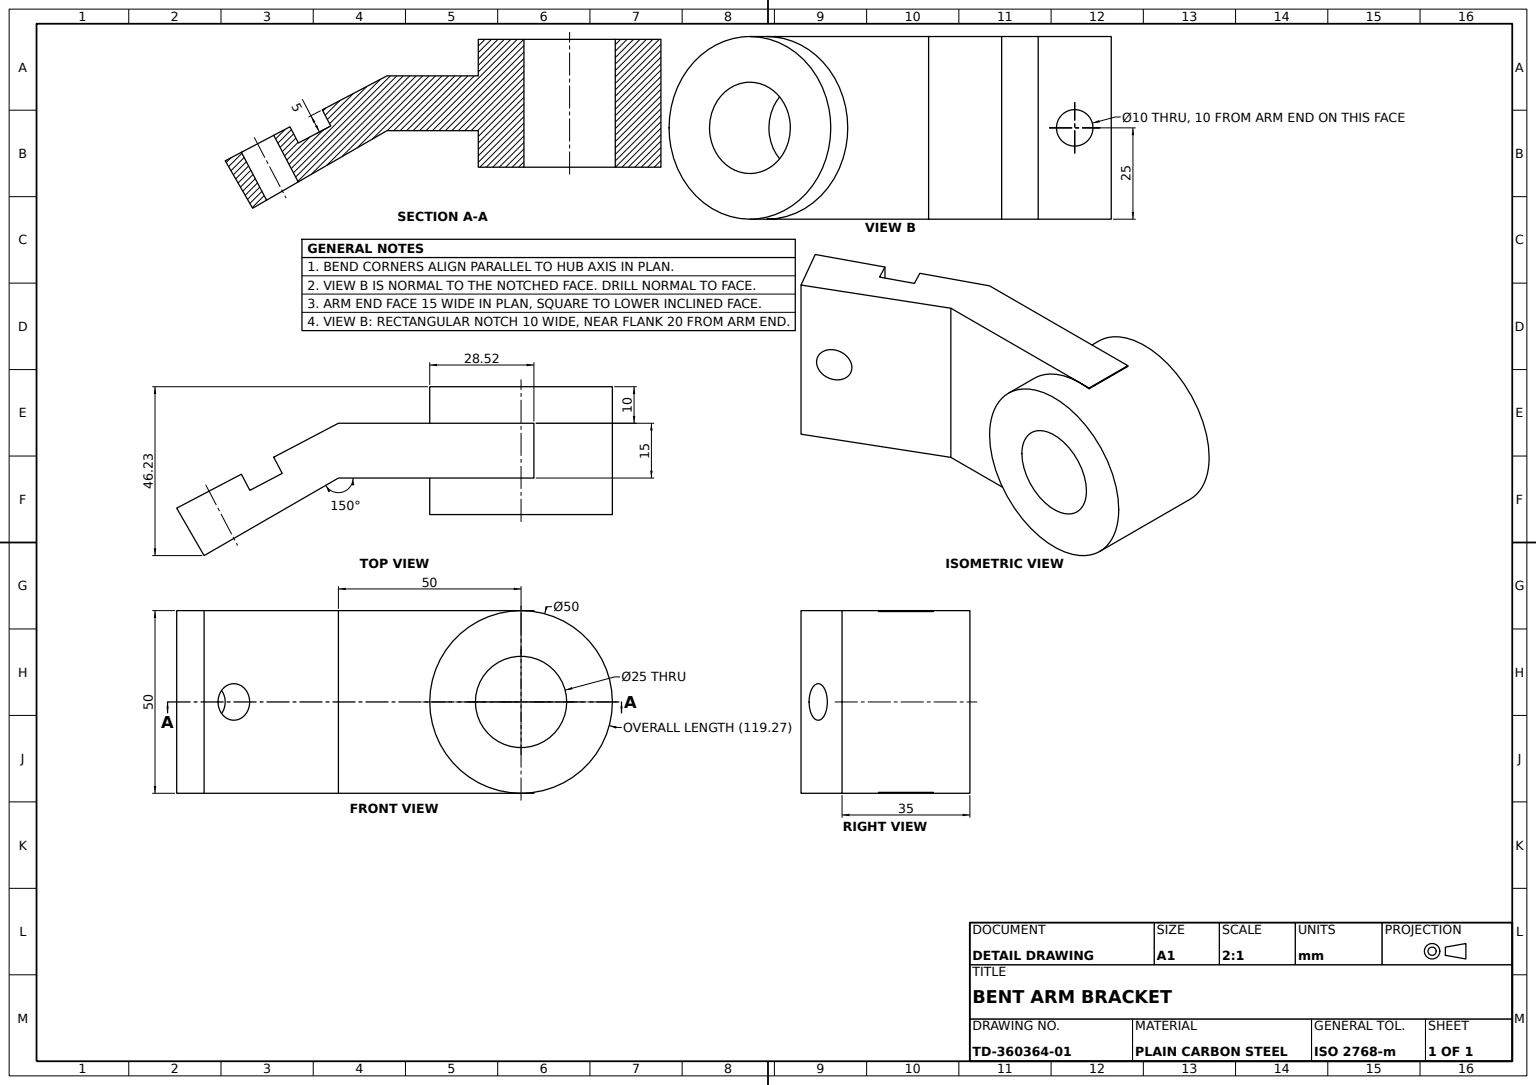
from build123d import *

# Parameters (mm, degrees)
HUB_TUBE_SKETCH_50_25_R   = 25
HUB_TUBE_SKETCH_50_25_R_2 = 12.5
HUB_TUBE_50_25_X35_DEPTH  = 17.5
ARM_50_DEPTH              = 25
TOP_NOTCH_CUT_DEPTH       = 111.509908397
CROSS_HOLE_SKETCH_10_R    = 5
CROSS_HOLE_10_DEPTH       = 101.657736852
BORE_CLEARANCE_CUT_DEPTH  = 108.931611768


with BuildPart() as part:
    # Hub Tube Sketch Ø50-Ø25 → Hub Tube Ø50-Ø25 x35 (new, symmetric)
    with BuildSketch(Plane.XY):
        Circle(HUB_TUBE_SKETCH_50_25_R)
        Circle(HUB_TUBE_SKETCH_50_25_R_2, mode=Mode.SUBTRACT)
    extrude(amount=HUB_TUBE_50_25_X35_DEPTH, both=True)

    # Arm Profile Sketch → Arm 50 (add, symmetric)
    with BuildSketch(Plane(origin=(0, 0, 0), x_dir=(1, 0, 0), z_dir=(0, 1, 0))):
        Polygon((3.520588359, 7.5), (-25, 7.5), (-50, 7.5), (-94.271090497, -15.73941794), (-86.771090497, -28.729798997), (-50, -7.5), (-25, -7.5), (3.520588359, -7.5), align=None)
    extrude(amount=ARM_50_DEPTH, both=True)

    # Top Notch Sketch → Top Notch Cut (cut, through all)
    with BuildSketch(Plane(origin=(0, 25, 0), x_dir=(1, 0, 0), z_dir=(0, 1, 0))):
        Polygon((-76.562654298, -6.443650764), (-74.238712504, -10.870759814), (-65.384494405, -6.222876226), (-67.708436199, -1.795767176), align=None)
    extrude(amount=-TOP_NOTCH_CUT_DEPTH, mode=Mode.SUBTRACT)

    # Cross Hole Sketch Ø10 → Cross Hole Ø10 (cut, through all)
    with BuildSketch(Plane(origin=(-13.887914048, 0, -26.456475856), x_dir=(-0.8854218099422658, 0, 0.46478835880275915), z_dir=(-0.46478835880275915, 0, -0.8854218099422658))):
        with Locations((80.785177806, 0)):
            Circle(CROSS_HOLE_SKETCH_10_R)
    extrude(amount=-CROSS_HOLE_10_DEPTH, mode=Mode.SUBTRACT)

    # Bore Clearance Sketch → Bore Clearance Cut (cut, through all)
    with BuildSketch(Plane(origin=(0, 0, -17.5), x_dir=(-1, 0, 0), z_dir=(0, 0, -1))):
        with BuildLine():
            Line((-3.520588359, 11.993975888), (-3.520588359, -11.993975888))
            ThreePointArc((-3.520588359, -11.993975888), (12.5, 0), (-3.520588359, 11.993975888))
        make_face()
    extrude(amount=-BORE_CLEARANCE_CUT_DEPTH, mode=Mode.SUBTRACT)


solid = part.part
